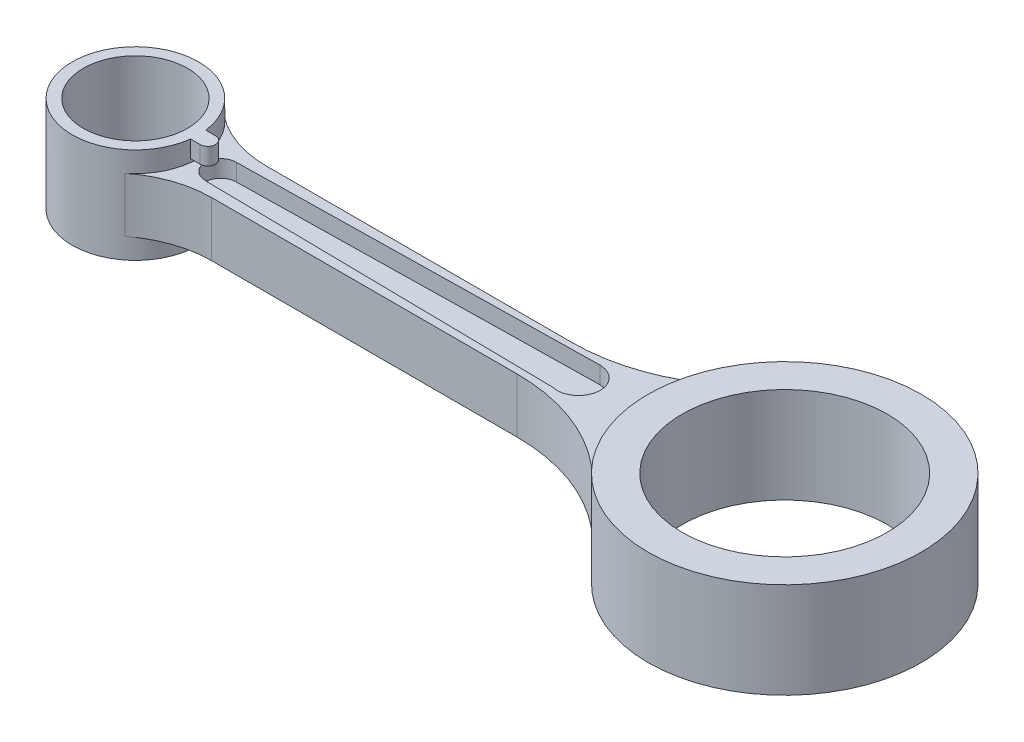
ISO-10303-21;
HEADER;
FILE_DESCRIPTION(('STEP AP214'),'2;1');
FILE_NAME('part.step','',(''),(''),'','','');
FILE_SCHEMA(('AUTOMOTIVE_DESIGN { 1 0 10303 214 1 1 1 1 }'));
ENDSEC;
DATA;
#1=APPLICATION_CONTEXT('core data for automotive mechanical design processes');
#2=APPLICATION_PROTOCOL_DEFINITION('international standard','automotive_design',2000,#1);
#3=PRODUCT_CONTEXT('',#1,'mechanical');
#4=PRODUCT('Part','Part','',(#3));
#5=PRODUCT_RELATED_PRODUCT_CATEGORY('part','',(#4));
#6=PRODUCT_DEFINITION_FORMATION('','',#4);
#7=PRODUCT_DEFINITION_CONTEXT('part definition',#1,'design');
#8=PRODUCT_DEFINITION('design','',#6,#7);
#9=PRODUCT_DEFINITION_SHAPE('','',#8);
#10=(LENGTH_UNIT() NAMED_UNIT(*) SI_UNIT(.MILLI.,.METRE.));
#11=(NAMED_UNIT(*) PLANE_ANGLE_UNIT() SI_UNIT($,.RADIAN.));
#12=(NAMED_UNIT(*) SI_UNIT($,.STERADIAN.) SOLID_ANGLE_UNIT());
#13=UNCERTAINTY_MEASURE_WITH_UNIT(LENGTH_MEASURE(1.E-05),#10,'distance_accuracy_value','');
#14=(GEOMETRIC_REPRESENTATION_CONTEXT(3) GLOBAL_UNCERTAINTY_ASSIGNED_CONTEXT((#13)) GLOBAL_UNIT_ASSIGNED_CONTEXT((#10,
#11,#12)) REPRESENTATION_CONTEXT('',''));
#15=CARTESIAN_POINT('',(0.,0.,0.));
#16=DIRECTION('',(0.,0.,1.));
#17=DIRECTION('',(1.,0.,0.));
#18=AXIS2_PLACEMENT_3D('',#15,#16,#17);
#19=CARTESIAN_POINT('',(12.3318325754668,7.,30.65));
#20=DIRECTION('',(0.,-1.,0.));
#21=DIRECTION('',(0.,0.,-1.));
#22=AXIS2_PLACEMENT_3D('',#19,#20,#21);
#23=CYLINDRICAL_SURFACE('',#22,26.65);
#24=DIRECTION('',(0.,1.,0.));
#25=VECTOR('',#24,1.);
#26=CARTESIAN_POINT('',(12.3318325754668,7.,4.));
#27=LINE('',#26,#25);
#28=CARTESIAN_POINT('',(12.3318325754668,-4.,4.));
#29=VERTEX_POINT('',#28);
#30=CARTESIAN_POINT('',(12.3318325754668,4.,4.));
#31=VERTEX_POINT('',#30);
#32=EDGE_CURVE('E337',#29,#31,#27,.T.);
#33=ORIENTED_EDGE('',*,*,#32,.F.);
#34=CARTESIAN_POINT('',(12.3318325754668,-4.,30.65));
#35=DIRECTION('',(0.,1.,0.));
#36=DIRECTION('',(0.,0.,1.));
#37=AXIS2_PLACEMENT_3D('',#34,#35,#36);
#38=CIRCLE('',#37,26.65);
#39=CARTESIAN_POINT('',(32.4225434407146,-4.,13.1404072883173));
#40=VERTEX_POINT('',#39);
#41=EDGE_CURVE('E341',#29,#40,#38,.F.);
#42=ORIENTED_EDGE('',*,*,#41,.T.);
#43=DIRECTION('',(0.,-1.,0.));
#44=VECTOR('',#43,1.);
#45=CARTESIAN_POINT('',(32.4225434407146,7.,13.1404072883173));
#46=LINE('',#45,#44);
#47=CARTESIAN_POINT('',(32.4225434407146,4.,13.1404072883173));
#48=VERTEX_POINT('',#47);
#49=EDGE_CURVE('E339',#48,#40,#46,.T.);
#50=ORIENTED_EDGE('',*,*,#49,.F.);
#51=CARTESIAN_POINT('',(12.3318325754668,4.,30.65));
#52=DIRECTION('',(0.,1.,0.));
#53=DIRECTION('',(0.,0.,1.));
#54=AXIS2_PLACEMENT_3D('',#51,#52,#53);
#55=CIRCLE('',#54,26.65);
#56=EDGE_CURVE('E48',#48,#31,#55,.T.);
#57=ORIENTED_EDGE('',*,*,#56,.T.);
#58=EDGE_LOOP('',(#33,#42,#50,#57));
#59=FACE_BOUND('',#58,.T.);
#60=ADVANCED_FACE('F41',(#59),#23,.F.);
#61=CARTESIAN_POINT('',(-32.3445554337723,7.,19.25));
#62=DIRECTION('',(0.,-1.,0.));
#63=DIRECTION('',(0.,0.,-1.));
#64=AXIS2_PLACEMENT_3D('',#61,#62,#63);
#65=CYLINDRICAL_SURFACE('',#64,15.25);
#66=DIRECTION('',(0.,-1.,0.));
#67=VECTOR('',#66,1.);
#68=CARTESIAN_POINT('',(-41.7780464392814,7.,7.26785714285715));
#69=LINE('',#68,#67);
#70=CARTESIAN_POINT('',(-41.7780464392814,-4.,7.26785714285715));
#71=VERTEX_POINT('',#70);
#72=CARTESIAN_POINT('',(-41.7780464392814,4.,7.26785714285715));
#73=VERTEX_POINT('',#72);
#74=EDGE_CURVE('E322',#71,#73,#69,.F.);
#75=ORIENTED_EDGE('',*,*,#74,.F.);
#76=CARTESIAN_POINT('',(-32.3445554337723,-4.,19.25));
#77=DIRECTION('',(0.,1.,0.));
#78=DIRECTION('',(0.,0.,1.));
#79=AXIS2_PLACEMENT_3D('',#76,#77,#78);
#80=CIRCLE('',#79,15.25);
#81=CARTESIAN_POINT('',(-32.3445554337723,-4.,4.));
#82=VERTEX_POINT('',#81);
#83=EDGE_CURVE('E334',#71,#82,#80,.F.);
#84=ORIENTED_EDGE('',*,*,#83,.T.);
#85=DIRECTION('',(0.,1.,0.));
#86=VECTOR('',#85,1.);
#87=CARTESIAN_POINT('',(-32.3445554337723,7.,4.));
#88=LINE('',#87,#86);
#89=CARTESIAN_POINT('',(-32.3445554337723,4.,4.));
#90=VERTEX_POINT('',#89);
#91=EDGE_CURVE('E330',#90,#82,#88,.F.);
#92=ORIENTED_EDGE('',*,*,#91,.F.);
#93=CARTESIAN_POINT('',(-32.3445554337723,4.,19.25));
#94=DIRECTION('',(0.,1.,0.));
#95=DIRECTION('',(0.,0.,1.));
#96=AXIS2_PLACEMENT_3D('',#93,#94,#95);
#97=CIRCLE('',#96,15.25);
#98=EDGE_CURVE('E335',#90,#73,#97,.T.);
#99=ORIENTED_EDGE('',*,*,#98,.T.);
#100=EDGE_LOOP('',(#75,#84,#92,#99));
#101=FACE_BOUND('',#100,.T.);
#102=ADVANCED_FACE('F356',(#101),#65,.F.);
#103=CARTESIAN_POINT('',(-32.3445554337723,7.,-19.25));
#104=DIRECTION('',(0.,-1.,0.));
#105=DIRECTION('',(0.,0.,-1.));
#106=AXIS2_PLACEMENT_3D('',#103,#104,#105);
#107=CYLINDRICAL_SURFACE('',#106,15.25);
#108=DIRECTION('',(0.,-1.,0.));
#109=VECTOR('',#108,1.);
#110=CARTESIAN_POINT('',(-41.7780464392814,7.,-7.26785714285714));
#111=LINE('',#110,#109);
#112=CARTESIAN_POINT('',(-41.7780464392814,4.,-7.26785714285714));
#113=VERTEX_POINT('',#112);
#114=CARTESIAN_POINT('',(-41.7780464392814,-4.,-7.26785714285714));
#115=VERTEX_POINT('',#114);
#116=EDGE_CURVE('E313',#113,#115,#111,.T.);
#117=ORIENTED_EDGE('',*,*,#116,.F.);
#118=CARTESIAN_POINT('',(-32.3445554337723,4.,-19.25));
#119=DIRECTION('',(0.,1.,0.));
#120=DIRECTION('',(0.,0.,1.));
#121=AXIS2_PLACEMENT_3D('',#118,#119,#120);
#122=CIRCLE('',#121,15.25);
#123=CARTESIAN_POINT('',(-32.3445554337723,4.,-4.));
#124=VERTEX_POINT('',#123);
#125=EDGE_CURVE('E318',#113,#124,#122,.T.);
#126=ORIENTED_EDGE('',*,*,#125,.T.);
#127=DIRECTION('',(0.,1.,0.));
#128=VECTOR('',#127,1.);
#129=CARTESIAN_POINT('',(-32.3445554337723,7.,-4.));
#130=LINE('',#129,#128);
#131=CARTESIAN_POINT('',(-32.3445554337723,-4.,-4.));
#132=VERTEX_POINT('',#131);
#133=EDGE_CURVE('E320',#132,#124,#130,.T.);
#134=ORIENTED_EDGE('',*,*,#133,.F.);
#135=CARTESIAN_POINT('',(-32.3445554337723,-4.,-19.25));
#136=DIRECTION('',(0.,1.,0.));
#137=DIRECTION('',(0.,0.,1.));
#138=AXIS2_PLACEMENT_3D('',#135,#136,#137);
#139=CIRCLE('',#138,15.25);
#140=EDGE_CURVE('E321',#132,#115,#139,.F.);
#141=ORIENTED_EDGE('',*,*,#140,.T.);
#142=EDGE_LOOP('',(#117,#126,#134,#141));
#143=FACE_BOUND('',#142,.T.);
#144=ADVANCED_FACE('F380',(#143),#107,.F.);
#145=CARTESIAN_POINT('',(12.3318325754668,7.,-30.65));
#146=DIRECTION('',(0.,-1.,0.));
#147=DIRECTION('',(0.,0.,-1.));
#148=AXIS2_PLACEMENT_3D('',#145,#146,#147);
#149=CYLINDRICAL_SURFACE('',#148,26.65);
#150=DIRECTION('',(0.,1.,0.));
#151=VECTOR('',#150,1.);
#152=CARTESIAN_POINT('',(12.3318325754668,7.,-4.));
#153=LINE('',#152,#151);
#154=CARTESIAN_POINT('',(12.3318325754668,4.,-4.));
#155=VERTEX_POINT('',#154);
#156=CARTESIAN_POINT('',(12.3318325754668,-4.,-4.));
#157=VERTEX_POINT('',#156);
#158=EDGE_CURVE('E303',#155,#157,#153,.F.);
#159=ORIENTED_EDGE('',*,*,#158,.F.);
#160=CARTESIAN_POINT('',(12.3318325754668,4.,-30.65));
#161=DIRECTION('',(0.,1.,0.));
#162=DIRECTION('',(0.,0.,1.));
#163=AXIS2_PLACEMENT_3D('',#160,#161,#162);
#164=CIRCLE('',#163,26.65);
#165=CARTESIAN_POINT('',(32.4225434407146,4.,-13.1404072883173));
#166=VERTEX_POINT('',#165);
#167=EDGE_CURVE('E307',#155,#166,#164,.T.);
#168=ORIENTED_EDGE('',*,*,#167,.T.);
#169=DIRECTION('',(0.,-1.,0.));
#170=VECTOR('',#169,1.);
#171=CARTESIAN_POINT('',(32.4225434407146,7.,-13.1404072883173));
#172=LINE('',#171,#170);
#173=CARTESIAN_POINT('',(32.4225434407146,-4.,-13.1404072883173));
#174=VERTEX_POINT('',#173);
#175=EDGE_CURVE('E306',#174,#166,#172,.F.);
#176=ORIENTED_EDGE('',*,*,#175,.F.);
#177=CARTESIAN_POINT('',(12.3318325754668,-4.,-30.65));
#178=DIRECTION('',(0.,1.,0.));
#179=DIRECTION('',(0.,0.,1.));
#180=AXIS2_PLACEMENT_3D('',#177,#178,#179);
#181=CIRCLE('',#180,26.65);
#182=EDGE_CURVE('E315',#174,#157,#181,.F.);
#183=ORIENTED_EDGE('',*,*,#182,.T.);
#184=EDGE_LOOP('',(#159,#168,#176,#183));
#185=FACE_BOUND('',#184,.T.);
#186=ADVANCED_FACE('F367',(#185),#149,.F.);
#187=CARTESIAN_POINT('',(-38.3065183264543,4.,4.));
#188=DIRECTION('',(0.,0.,-1.));
#189=DIRECTION('',(-1.,0.,0.));
#190=AXIS2_PLACEMENT_3D('',#187,#188,#189);
#191=PLANE('',#190);
#192=DIRECTION('',(1.,0.,0.));
#193=VECTOR('',#192,1.);
#194=CARTESIAN_POINT('',(-38.3065183264543,-4.,4.));
#195=LINE('',#194,#193);
#196=EDGE_CURVE('E271',#82,#29,#195,.T.);
#197=ORIENTED_EDGE('',*,*,#196,.T.);
#198=ORIENTED_EDGE('',*,*,#32,.T.);
#199=DIRECTION('',(1.,0.,0.));
#200=VECTOR('',#199,1.);
#201=CARTESIAN_POINT('',(-39.3751793252666,4.,4.));
#202=LINE('',#201,#200);
#203=EDGE_CURVE('E274',#90,#31,#202,.T.);
#204=ORIENTED_EDGE('',*,*,#203,.F.);
#205=ORIENTED_EDGE('',*,*,#91,.T.);
#206=EDGE_LOOP('',(#197,#198,#204,#205));
#207=FACE_BOUND('',#206,.T.);
#208=ADVANCED_FACE('F354',(#207),#191,.F.);
#209=CARTESIAN_POINT('',(27.2825504756529,4.,-4.));
#210=DIRECTION('',(0.,0.,1.));
#211=DIRECTION('',(1.,0.,0.));
#212=AXIS2_PLACEMENT_3D('',#209,#210,#211);
#213=PLANE('',#212);
#214=DIRECTION('',(-1.,0.,0.));
#215=VECTOR('',#214,1.);
#216=CARTESIAN_POINT('',(27.2825504756529,-4.,-4.));
#217=LINE('',#216,#215);
#218=EDGE_CURVE('E280',#157,#132,#217,.T.);
#219=ORIENTED_EDGE('',*,*,#218,.T.);
#220=ORIENTED_EDGE('',*,*,#133,.T.);
#221=DIRECTION('',(-1.,0.,0.));
#222=VECTOR('',#221,1.);
#223=CARTESIAN_POINT('',(27.2825504756529,4.,-4.));
#224=LINE('',#223,#222);
#225=EDGE_CURVE('E276',#155,#124,#224,.T.);
#226=ORIENTED_EDGE('',*,*,#225,.F.);
#227=ORIENTED_EDGE('',*,*,#158,.T.);
#228=EDGE_LOOP('',(#219,#220,#226,#227));
#229=FACE_BOUND('',#228,.T.);
#230=ADVANCED_FACE('F373',(#229),#213,.F.);
#231=CARTESIAN_POINT('',(47.5,7.,0.));
#232=DIRECTION('',(0.,-1.,0.));
#233=DIRECTION('',(0.,0.,-1.));
#234=AXIS2_PLACEMENT_3D('',#231,#232,#233);
#235=CYLINDRICAL_SURFACE('',#234,15.);
#236=CARTESIAN_POINT('',(47.5,7.,0.));
#237=DIRECTION('',(0.,1.,0.));
#238=DIRECTION('',(0.,0.,1.));
#239=AXIS2_PLACEMENT_3D('',#236,#237,#238);
#240=CIRCLE('',#239,15.);
#241=CARTESIAN_POINT('',(47.5,7.,15.));
#242=VERTEX_POINT('',#241);
#243=EDGE_CURVE('E289',#242,#242,#240,.T.);
#244=ORIENTED_EDGE('',*,*,#243,.T.);
#245=EDGE_LOOP('',(#244));
#246=FACE_BOUND('',#245,.T.);
#247=CARTESIAN_POINT('',(47.5,-7.,0.));
#248=DIRECTION('',(0.,1.,0.));
#249=DIRECTION('',(0.,0.,1.));
#250=AXIS2_PLACEMENT_3D('',#247,#248,#249);
#251=CIRCLE('',#250,15.);
#252=CARTESIAN_POINT('',(47.5,-7.,15.));
#253=VERTEX_POINT('',#252);
#254=EDGE_CURVE('E282',#253,#253,#251,.T.);
#255=ORIENTED_EDGE('',*,*,#254,.F.);
#256=EDGE_LOOP('',(#255));
#257=FACE_BOUND('',#256,.T.);
#258=ADVANCED_FACE('F411',(#246,#257),#235,.F.);
#259=CARTESIAN_POINT('',(47.5,7.,0.));
#260=DIRECTION('',(0.,-1.,0.));
#261=DIRECTION('',(0.,0.,-1.));
#262=AXIS2_PLACEMENT_3D('',#259,#260,#261);
#263=CYLINDRICAL_SURFACE('',#262,20.);
#264=ORIENTED_EDGE('',*,*,#49,.T.);
#265=CARTESIAN_POINT('',(47.5,-4.,0.));
#266=DIRECTION('',(0.,1.,0.));
#267=DIRECTION('',(0.,0.,1.));
#268=AXIS2_PLACEMENT_3D('',#265,#266,#267);
#269=CIRCLE('',#268,20.);
#270=EDGE_CURVE('E291',#174,#40,#269,.T.);
#271=ORIENTED_EDGE('',*,*,#270,.F.);
#272=ORIENTED_EDGE('',*,*,#175,.T.);
#273=CARTESIAN_POINT('',(47.5,4.,0.));
#274=DIRECTION('',(0.,1.,0.));
#275=DIRECTION('',(0.,0.,1.));
#276=AXIS2_PLACEMENT_3D('',#273,#274,#275);
#277=CIRCLE('',#276,20.);
#278=EDGE_CURVE('E299',#166,#48,#277,.T.);
#279=ORIENTED_EDGE('',*,*,#278,.T.);
#280=EDGE_LOOP('',(#264,#271,#272,#279));
#281=FACE_BOUND('',#280,.T.);
#282=CARTESIAN_POINT('',(47.5,7.,0.));
#283=DIRECTION('',(0.,1.,0.));
#284=DIRECTION('',(0.,0.,1.));
#285=AXIS2_PLACEMENT_3D('',#282,#283,#284);
#286=CIRCLE('',#285,20.);
#287=CARTESIAN_POINT('',(47.5,7.,20.));
#288=VERTEX_POINT('',#287);
#289=EDGE_CURVE('E288',#288,#288,#286,.T.);
#290=ORIENTED_EDGE('',*,*,#289,.F.);
#291=EDGE_LOOP('',(#290));
#292=FACE_BOUND('',#291,.T.);
#293=CARTESIAN_POINT('',(47.5,-7.,0.));
#294=DIRECTION('',(0.,1.,0.));
#295=DIRECTION('',(0.,0.,1.));
#296=AXIS2_PLACEMENT_3D('',#293,#294,#295);
#297=CIRCLE('',#296,20.);
#298=CARTESIAN_POINT('',(47.5,-7.,20.));
#299=VERTEX_POINT('',#298);
#300=EDGE_CURVE('E287',#299,#299,#297,.T.);
#301=ORIENTED_EDGE('',*,*,#300,.T.);
#302=EDGE_LOOP('',(#301));
#303=FACE_BOUND('',#302,.T.);
#304=ADVANCED_FACE('F364',(#281,#292,#303),#263,.T.);
#305=CARTESIAN_POINT('',(0.,7.,0.));
#306=DIRECTION('',(0.,1.,0.));
#307=DIRECTION('',(0.,0.,1.));
#308=AXIS2_PLACEMENT_3D('',#305,#306,#307);
#309=PLANE('',#308);
#310=ORIENTED_EDGE('',*,*,#243,.F.);
#311=EDGE_LOOP('',(#310));
#312=FACE_BOUND('',#311,.T.);
#313=ORIENTED_EDGE('',*,*,#289,.T.);
#314=EDGE_LOOP('',(#313));
#315=FACE_BOUND('',#314,.T.);
#316=ADVANCED_FACE('F417',(#312,#315),#309,.T.);
#317=CARTESIAN_POINT('',(0.,-7.,0.));
#318=DIRECTION('',(0.,1.,0.));
#319=DIRECTION('',(0.,0.,1.));
#320=AXIS2_PLACEMENT_3D('',#317,#318,#319);
#321=PLANE('',#320);
#322=ORIENTED_EDGE('',*,*,#254,.T.);
#323=EDGE_LOOP('',(#322));
#324=FACE_BOUND('',#323,.T.);
#325=ORIENTED_EDGE('',*,*,#300,.F.);
#326=EDGE_LOOP('',(#325));
#327=FACE_BOUND('',#326,.T.);
#328=ADVANCED_FACE('F423',(#324,#327),#321,.F.);
#329=CARTESIAN_POINT('',(0.,4.,0.));
#330=DIRECTION('',(0.,1.,0.));
#331=DIRECTION('',(0.,0.,1.));
#332=AXIS2_PLACEMENT_3D('',#329,#330,#331);
#333=PLANE('',#332);
#334=DIRECTION('',(0.999892618853564,0.,0.0146543768943431));
#335=VECTOR('',#334,1.);
#336=CARTESIAN_POINT('',(-0.0414886671393151,4.,2.8308410748387));
#337=LINE('',#336,#335);
#338=CARTESIAN_POINT('',(-35.01,4.,2.31834429784139));
#339=VERTEX_POINT('',#338);
#340=CARTESIAN_POINT('',(16.5719942554758,4.,3.07432746096172));
#341=VERTEX_POINT('',#340);
#342=EDGE_CURVE('E65',#339,#341,#337,.T.);
#343=ORIENTED_EDGE('',*,*,#342,.F.);
#344=DIRECTION('',(0.,0.,1.));
#345=VECTOR('',#344,1.);
#346=CARTESIAN_POINT('',(-35.01,4.,0.));
#347=LINE('',#346,#345);
#348=CARTESIAN_POINT('',(-35.01,4.,2.27758375371882));
#349=VERTEX_POINT('',#348);
#350=EDGE_CURVE('E208',#349,#339,#347,.T.);
#351=ORIENTED_EDGE('',*,*,#350,.F.);
#352=CARTESIAN_POINT('',(-35.01,4.,0.));
#353=DIRECTION('',(0.,1.,0.));
#354=DIRECTION('',(0.,0.,1.));
#355=AXIS2_PLACEMENT_3D('',#352,#353,#354);
#356=CIRCLE('',#355,2.27758375371882);
#357=CARTESIAN_POINT('',(-35.01,4.,-2.27758375371881));
#358=VERTEX_POINT('',#357);
#359=EDGE_CURVE('E245',#358,#349,#356,.T.);
#360=ORIENTED_EDGE('',*,*,#359,.F.);
#361=DIRECTION('',(0.,0.,1.));
#362=VECTOR('',#361,1.);
#363=CARTESIAN_POINT('',(-35.01,4.,0.));
#364=LINE('',#363,#362);
#365=CARTESIAN_POINT('',(-35.01,4.,-2.28421044966346));
#366=VERTEX_POINT('',#365);
#367=EDGE_CURVE('E237',#366,#358,#364,.T.);
#368=ORIENTED_EDGE('',*,*,#367,.F.);
#369=DIRECTION('',(-0.99985003095603,0.,0.0173180714060757));
#370=VECTOR('',#369,1.);
#371=CARTESIAN_POINT('',(-0.0500522322392675,4.,-2.8897401321658));
#372=LINE('',#371,#370);
#373=CARTESIAN_POINT('',(17.33,4.,-3.19077426356593));
#374=VERTEX_POINT('',#373);
#375=EDGE_CURVE('E236',#374,#366,#372,.T.);
#376=ORIENTED_EDGE('',*,*,#375,.F.);
#377=DIRECTION('',(0.,0.,-1.));
#378=VECTOR('',#377,1.);
#379=CARTESIAN_POINT('',(17.33,4.,0.));
#380=LINE('',#379,#378);
#381=CARTESIAN_POINT('',(17.33,4.,-3.1663957500532));
#382=VERTEX_POINT('',#381);
#383=EDGE_CURVE('E231',#382,#374,#380,.T.);
#384=ORIENTED_EDGE('',*,*,#383,.F.);
#385=CARTESIAN_POINT('',(17.33,4.,0.));
#386=DIRECTION('',(0.,1.,0.));
#387=DIRECTION('',(0.,0.,1.));
#388=AXIS2_PLACEMENT_3D('',#385,#386,#387);
#389=CIRCLE('',#388,3.1663957500532);
#390=EDGE_CURVE('E229',#341,#382,#389,.T.);
#391=ORIENTED_EDGE('',*,*,#390,.F.);
#392=EDGE_LOOP('',(#343,#351,#360,#368,#376,#384,#391));
#393=FACE_BOUND('',#392,.T.);
#394=ORIENTED_EDGE('',*,*,#278,.F.);
#395=ORIENTED_EDGE('',*,*,#167,.F.);
#396=ORIENTED_EDGE('',*,*,#225,.T.);
#397=ORIENTED_EDGE('',*,*,#125,.F.);
#398=CARTESIAN_POINT('',(-47.5,4.,0.));
#399=DIRECTION('',(0.,1.,0.));
#400=DIRECTION('',(0.,0.,1.));
#401=AXIS2_PLACEMENT_3D('',#398,#399,#400);
#402=CIRCLE('',#401,9.25);
#403=EDGE_CURVE('E266',#113,#73,#402,.F.);
#404=ORIENTED_EDGE('',*,*,#403,.T.);
#405=ORIENTED_EDGE('',*,*,#98,.F.);
#406=ORIENTED_EDGE('',*,*,#203,.T.);
#407=ORIENTED_EDGE('',*,*,#56,.F.);
#408=EDGE_LOOP('',(#394,#395,#396,#397,#404,#405,#406,#407));
#409=FACE_BOUND('',#408,.T.);
#410=ADVANCED_FACE('F355',(#393,#409),#333,.T.);
#411=CARTESIAN_POINT('',(0.,-4.,0.));
#412=DIRECTION('',(0.,1.,0.));
#413=DIRECTION('',(0.,0.,1.));
#414=AXIS2_PLACEMENT_3D('',#411,#412,#413);
#415=PLANE('',#414);
#416=CARTESIAN_POINT('',(-47.5,-4.,0.));
#417=DIRECTION('',(0.,1.,0.));
#418=DIRECTION('',(0.,0.,1.));
#419=AXIS2_PLACEMENT_3D('',#416,#417,#418);
#420=CIRCLE('',#419,9.25);
#421=EDGE_CURVE('E301',#115,#71,#420,.F.);
#422=ORIENTED_EDGE('',*,*,#421,.F.);
#423=ORIENTED_EDGE('',*,*,#140,.F.);
#424=ORIENTED_EDGE('',*,*,#218,.F.);
#425=ORIENTED_EDGE('',*,*,#182,.F.);
#426=ORIENTED_EDGE('',*,*,#270,.T.);
#427=ORIENTED_EDGE('',*,*,#41,.F.);
#428=ORIENTED_EDGE('',*,*,#196,.F.);
#429=ORIENTED_EDGE('',*,*,#83,.F.);
#430=EDGE_LOOP('',(#422,#423,#424,#425,#426,#427,#428,#429));
#431=FACE_BOUND('',#430,.T.);
#432=ADVANCED_FACE('F363',(#431),#415,.F.);
#433=CARTESIAN_POINT('',(-47.5,7.,0.));
#434=DIRECTION('',(0.,-1.,0.));
#435=DIRECTION('',(0.,0.,-1.));
#436=AXIS2_PLACEMENT_3D('',#433,#434,#435);
#437=CYLINDRICAL_SURFACE('',#436,7.625);
#438=CARTESIAN_POINT('',(-47.5,7.,0.));
#439=DIRECTION('',(0.,1.,0.));
#440=DIRECTION('',(0.,0.,1.));
#441=AXIS2_PLACEMENT_3D('',#438,#439,#440);
#442=CIRCLE('',#441,7.625);
#443=CARTESIAN_POINT('',(-47.5,7.,7.62500000000001));
#444=VERTEX_POINT('',#443);
#445=EDGE_CURVE('E262',#444,#444,#442,.T.);
#446=ORIENTED_EDGE('',*,*,#445,.T.);
#447=EDGE_LOOP('',(#446));
#448=FACE_BOUND('',#447,.T.);
#449=CARTESIAN_POINT('',(-47.5,-7.,0.));
#450=DIRECTION('',(0.,1.,0.));
#451=DIRECTION('',(0.,0.,1.));
#452=AXIS2_PLACEMENT_3D('',#449,#450,#451);
#453=CIRCLE('',#452,7.625);
#454=CARTESIAN_POINT('',(-47.5,-7.,7.62500000000001));
#455=VERTEX_POINT('',#454);
#456=EDGE_CURVE('E248',#455,#455,#453,.T.);
#457=ORIENTED_EDGE('',*,*,#456,.F.);
#458=EDGE_LOOP('',(#457));
#459=FACE_BOUND('',#458,.T.);
#460=ADVANCED_FACE('F384',(#448,#459),#437,.F.);
#461=CARTESIAN_POINT('',(-47.5,7.,0.));
#462=DIRECTION('',(0.,-1.,0.));
#463=DIRECTION('',(0.,0.,-1.));
#464=AXIS2_PLACEMENT_3D('',#461,#462,#463);
#465=CYLINDRICAL_SURFACE('',#464,9.25);
#466=CARTESIAN_POINT('',(-47.5,7.,0.));
#467=DIRECTION('',(0.,1.,0.));
#468=DIRECTION('',(0.,0.,1.));
#469=AXIS2_PLACEMENT_3D('',#466,#467,#468);
#470=CIRCLE('',#469,9.25);
#471=CARTESIAN_POINT('',(-38.3174472503557,7.,-1.115));
#472=VERTEX_POINT('',#471);
#473=CARTESIAN_POINT('',(-38.3174472503557,7.,1.115));
#474=VERTEX_POINT('',#473);
#475=EDGE_CURVE('E261',#472,#474,#470,.T.);
#476=ORIENTED_EDGE('',*,*,#475,.F.);
#477=DIRECTION('',(0.,-1.,0.));
#478=VECTOR('',#477,1.);
#479=CARTESIAN_POINT('',(-38.3174472503557,7.,-1.115));
#480=LINE('',#479,#478);
#481=CARTESIAN_POINT('',(-38.3174472503557,4.5,-1.115));
#482=VERTEX_POINT('',#481);
#483=EDGE_CURVE('E205',#472,#482,#480,.T.);
#484=ORIENTED_EDGE('',*,*,#483,.T.);
#485=CARTESIAN_POINT('',(-47.5,4.5,0.));
#486=DIRECTION('',(0.,1.,0.));
#487=DIRECTION('',(0.,0.,1.));
#488=AXIS2_PLACEMENT_3D('',#485,#486,#487);
#489=CIRCLE('',#488,9.25);
#490=CARTESIAN_POINT('',(-38.3174472503557,4.5,1.115));
#491=VERTEX_POINT('',#490);
#492=EDGE_CURVE('E11',#491,#482,#489,.T.);
#493=ORIENTED_EDGE('',*,*,#492,.F.);
#494=DIRECTION('',(0.,-1.,0.));
#495=VECTOR('',#494,1.);
#496=CARTESIAN_POINT('',(-38.3174472503557,7.,1.115));
#497=LINE('',#496,#495);
#498=EDGE_CURVE('E178',#491,#474,#497,.F.);
#499=ORIENTED_EDGE('',*,*,#498,.T.);
#500=EDGE_LOOP('',(#476,#484,#493,#499));
#501=FACE_BOUND('',#500,.T.);
#502=ORIENTED_EDGE('',*,*,#421,.T.);
#503=ORIENTED_EDGE('',*,*,#74,.T.);
#504=ORIENTED_EDGE('',*,*,#403,.F.);
#505=ORIENTED_EDGE('',*,*,#116,.T.);
#506=EDGE_LOOP('',(#502,#503,#504,#505));
#507=FACE_BOUND('',#506,.T.);
#508=CARTESIAN_POINT('',(-47.5,-7.,0.));
#509=DIRECTION('',(0.,1.,0.));
#510=DIRECTION('',(0.,0.,1.));
#511=AXIS2_PLACEMENT_3D('',#508,#509,#510);
#512=CIRCLE('',#511,9.25);
#513=CARTESIAN_POINT('',(-47.5,-7.,9.25000000000001));
#514=VERTEX_POINT('',#513);
#515=EDGE_CURVE('E263',#514,#514,#512,.T.);
#516=ORIENTED_EDGE('',*,*,#515,.T.);
#517=EDGE_LOOP('',(#516));
#518=FACE_BOUND('',#517,.T.);
#519=ADVANCED_FACE('F378',(#501,#507,#518),#465,.T.);
#520=CARTESIAN_POINT('',(0.,7.,0.));
#521=DIRECTION('',(0.,1.,0.));
#522=DIRECTION('',(0.,0.,1.));
#523=AXIS2_PLACEMENT_3D('',#520,#521,#522);
#524=PLANE('',#523);
#525=ORIENTED_EDGE('',*,*,#475,.T.);
#526=DIRECTION('',(1.,0.,0.));
#527=VECTOR('',#526,1.);
#528=CARTESIAN_POINT('',(0.,7.,1.115));
#529=LINE('',#528,#527);
#530=CARTESIAN_POINT('',(-36.9060551700783,7.,1.115));
#531=VERTEX_POINT('',#530);
#532=EDGE_CURVE('E199',#474,#531,#529,.T.);
#533=ORIENTED_EDGE('',*,*,#532,.T.);
#534=CARTESIAN_POINT('',(-36.9060551700783,7.,0.));
#535=DIRECTION('',(0.,1.,0.));
#536=DIRECTION('',(0.,0.,1.));
#537=AXIS2_PLACEMENT_3D('',#534,#535,#536);
#538=CIRCLE('',#537,1.115);
#539=CARTESIAN_POINT('',(-36.9060551700783,7.,-1.115));
#540=VERTEX_POINT('',#539);
#541=EDGE_CURVE('E189',#531,#540,#538,.T.);
#542=ORIENTED_EDGE('',*,*,#541,.T.);
#543=DIRECTION('',(-1.,0.,0.));
#544=VECTOR('',#543,1.);
#545=CARTESIAN_POINT('',(0.,7.,-1.115));
#546=LINE('',#545,#544);
#547=EDGE_CURVE('E54',#540,#472,#546,.T.);
#548=ORIENTED_EDGE('',*,*,#547,.T.);
#549=EDGE_LOOP('',(#525,#533,#542,#548));
#550=FACE_BOUND('',#549,.T.);
#551=ORIENTED_EDGE('',*,*,#445,.F.);
#552=EDGE_LOOP('',(#551));
#553=FACE_BOUND('',#552,.T.);
#554=ADVANCED_FACE('F385',(#550,#553),#524,.T.);
#555=CARTESIAN_POINT('',(0.,-7.,0.));
#556=DIRECTION('',(0.,1.,0.));
#557=DIRECTION('',(0.,0.,1.));
#558=AXIS2_PLACEMENT_3D('',#555,#556,#557);
#559=PLANE('',#558);
#560=ORIENTED_EDGE('',*,*,#456,.T.);
#561=EDGE_LOOP('',(#560));
#562=FACE_BOUND('',#561,.T.);
#563=ORIENTED_EDGE('',*,*,#515,.F.);
#564=EDGE_LOOP('',(#563));
#565=FACE_BOUND('',#564,.T.);
#566=ADVANCED_FACE('F390',(#562,#565),#559,.F.);
#567=CARTESIAN_POINT('',(-0.0414886671393151,1.5,2.8308410748387));
#568=DIRECTION('',(-0.0146543768943431,0.,0.999892618853564));
#569=DIRECTION('',(0.999892618853564,0.,0.0146543768943431));
#570=AXIS2_PLACEMENT_3D('',#567,#568,#569);
#571=PLANE('',#570);
#572=ORIENTED_EDGE('',*,*,#342,.T.);
#573=DIRECTION('',(0.,1.,0.));
#574=VECTOR('',#573,1.);
#575=CARTESIAN_POINT('',(16.5719942554758,1.5,3.07432746096172));
#576=LINE('',#575,#574);
#577=CARTESIAN_POINT('',(16.5719942554758,1.5,3.07432746096172));
#578=VERTEX_POINT('',#577);
#579=EDGE_CURVE('E226',#578,#341,#576,.T.);
#580=ORIENTED_EDGE('',*,*,#579,.F.);
#581=DIRECTION('',(0.999892618853564,0.,0.0146543768943431));
#582=VECTOR('',#581,1.);
#583=CARTESIAN_POINT('',(-0.0414886671393151,1.5,2.8308410748387));
#584=LINE('',#583,#582);
#585=CARTESIAN_POINT('',(-35.01,1.5,2.31834429784139));
#586=VERTEX_POINT('',#585);
#587=EDGE_CURVE('E207',#586,#578,#584,.T.);
#588=ORIENTED_EDGE('',*,*,#587,.F.);
#589=DIRECTION('',(0.,1.,0.));
#590=VECTOR('',#589,1.);
#591=CARTESIAN_POINT('',(-35.01,1.5,2.31834429784139));
#592=LINE('',#591,#590);
#593=EDGE_CURVE('E250',#586,#339,#592,.T.);
#594=ORIENTED_EDGE('',*,*,#593,.T.);
#595=EDGE_LOOP('',(#572,#580,#588,#594));
#596=FACE_BOUND('',#595,.T.);
#597=ADVANCED_FACE('F387',(#596),#571,.F.);
#598=CARTESIAN_POINT('',(-35.01,1.5,0.));
#599=DIRECTION('',(-1.,0.,0.));
#600=DIRECTION('',(0.,0.,1.));
#601=AXIS2_PLACEMENT_3D('',#598,#599,#600);
#602=PLANE('',#601);
#603=ORIENTED_EDGE('',*,*,#350,.T.);
#604=ORIENTED_EDGE('',*,*,#593,.F.);
#605=DIRECTION('',(0.,0.,1.));
#606=VECTOR('',#605,1.);
#607=CARTESIAN_POINT('',(-35.01,1.5,0.));
#608=LINE('',#607,#606);
#609=CARTESIAN_POINT('',(-35.01,1.5,2.27758375371882));
#610=VERTEX_POINT('',#609);
#611=EDGE_CURVE('E222',#610,#586,#608,.T.);
#612=ORIENTED_EDGE('',*,*,#611,.F.);
#613=DIRECTION('',(0.,1.,0.));
#614=VECTOR('',#613,1.);
#615=CARTESIAN_POINT('',(-35.01,1.5,2.27758375371882));
#616=LINE('',#615,#614);
#617=EDGE_CURVE('E249',#610,#349,#616,.T.);
#618=ORIENTED_EDGE('',*,*,#617,.T.);
#619=EDGE_LOOP('',(#603,#604,#612,#618));
#620=FACE_BOUND('',#619,.T.);
#621=ADVANCED_FACE('F400',(#620),#602,.F.);
#622=CARTESIAN_POINT('',(-35.01,1.5,0.));
#623=DIRECTION('',(0.,1.,0.));
#624=DIRECTION('',(0.,0.,1.));
#625=AXIS2_PLACEMENT_3D('',#622,#623,#624);
#626=CYLINDRICAL_SURFACE('',#625,2.27758375371882);
#627=ORIENTED_EDGE('',*,*,#359,.T.);
#628=ORIENTED_EDGE('',*,*,#617,.F.);
#629=CARTESIAN_POINT('',(-35.01,1.5,0.));
#630=DIRECTION('',(0.,1.,0.));
#631=DIRECTION('',(0.,0.,1.));
#632=AXIS2_PLACEMENT_3D('',#629,#630,#631);
#633=CIRCLE('',#632,2.27758375371882);
#634=CARTESIAN_POINT('',(-35.01,1.5,-2.27758375371881));
#635=VERTEX_POINT('',#634);
#636=EDGE_CURVE('E221',#635,#610,#633,.T.);
#637=ORIENTED_EDGE('',*,*,#636,.F.);
#638=DIRECTION('',(0.,1.,0.));
#639=VECTOR('',#638,1.);
#640=CARTESIAN_POINT('',(-35.01,1.5,-2.27758375371881));
#641=LINE('',#640,#639);
#642=EDGE_CURVE('E255',#635,#358,#641,.T.);
#643=ORIENTED_EDGE('',*,*,#642,.T.);
#644=EDGE_LOOP('',(#627,#628,#637,#643));
#645=FACE_BOUND('',#644,.T.);
#646=ADVANCED_FACE('F489',(#645),#626,.F.);
#647=CARTESIAN_POINT('',(-35.01,1.5,0.));
#648=DIRECTION('',(-1.,0.,0.));
#649=DIRECTION('',(0.,0.,1.));
#650=AXIS2_PLACEMENT_3D('',#647,#648,#649);
#651=PLANE('',#650);
#652=ORIENTED_EDGE('',*,*,#367,.T.);
#653=ORIENTED_EDGE('',*,*,#642,.F.);
#654=DIRECTION('',(0.,0.,1.));
#655=VECTOR('',#654,1.);
#656=CARTESIAN_POINT('',(-35.01,1.5,0.));
#657=LINE('',#656,#655);
#658=CARTESIAN_POINT('',(-35.01,1.5,-2.28421044966346));
#659=VERTEX_POINT('',#658);
#660=EDGE_CURVE('E216',#659,#635,#657,.T.);
#661=ORIENTED_EDGE('',*,*,#660,.F.);
#662=DIRECTION('',(0.,1.,0.));
#663=VECTOR('',#662,1.);
#664=CARTESIAN_POINT('',(-35.01,1.5,-2.28421044966346));
#665=LINE('',#664,#663);
#666=EDGE_CURVE('E251',#659,#366,#665,.T.);
#667=ORIENTED_EDGE('',*,*,#666,.T.);
#668=EDGE_LOOP('',(#652,#653,#661,#667));
#669=FACE_BOUND('',#668,.T.);
#670=ADVANCED_FACE('F497',(#669),#651,.F.);
#671=CARTESIAN_POINT('',(-0.0500522322392675,1.5,-2.8897401321658));
#672=DIRECTION('',(-0.0173180714060757,0.,-0.99985003095603));
#673=DIRECTION('',(-0.99985003095603,0.,0.0173180714060757));
#674=AXIS2_PLACEMENT_3D('',#671,#672,#673);
#675=PLANE('',#674);
#676=ORIENTED_EDGE('',*,*,#375,.T.);
#677=ORIENTED_EDGE('',*,*,#666,.F.);
#678=DIRECTION('',(-0.99985003095603,0.,0.0173180714060757));
#679=VECTOR('',#678,1.);
#680=CARTESIAN_POINT('',(-0.0500522322392675,1.5,-2.8897401321658));
#681=LINE('',#680,#679);
#682=CARTESIAN_POINT('',(17.33,1.5,-3.19077426356593));
#683=VERTEX_POINT('',#682);
#684=EDGE_CURVE('E217',#683,#659,#681,.T.);
#685=ORIENTED_EDGE('',*,*,#684,.F.);
#686=DIRECTION('',(0.,1.,0.));
#687=VECTOR('',#686,1.);
#688=CARTESIAN_POINT('',(17.33,1.5,-3.19077426356593));
#689=LINE('',#688,#687);
#690=EDGE_CURVE('E259',#683,#374,#689,.T.);
#691=ORIENTED_EDGE('',*,*,#690,.T.);
#692=EDGE_LOOP('',(#676,#677,#685,#691));
#693=FACE_BOUND('',#692,.T.);
#694=ADVANCED_FACE('F507',(#693),#675,.F.);
#695=CARTESIAN_POINT('',(17.33,1.5,0.));
#696=DIRECTION('',(1.,0.,0.));
#697=DIRECTION('',(0.,0.,-1.));
#698=AXIS2_PLACEMENT_3D('',#695,#696,#697);
#699=PLANE('',#698);
#700=ORIENTED_EDGE('',*,*,#383,.T.);
#701=ORIENTED_EDGE('',*,*,#690,.F.);
#702=DIRECTION('',(0.,0.,-1.));
#703=VECTOR('',#702,1.);
#704=CARTESIAN_POINT('',(17.33,1.5,0.));
#705=LINE('',#704,#703);
#706=CARTESIAN_POINT('',(17.33,1.5,-3.1663957500532));
#707=VERTEX_POINT('',#706);
#708=EDGE_CURVE('E215',#707,#683,#705,.T.);
#709=ORIENTED_EDGE('',*,*,#708,.F.);
#710=DIRECTION('',(0.,1.,0.));
#711=VECTOR('',#710,1.);
#712=CARTESIAN_POINT('',(17.33,1.5,-3.1663957500532));
#713=LINE('',#712,#711);
#714=EDGE_CURVE('E260',#707,#382,#713,.T.);
#715=ORIENTED_EDGE('',*,*,#714,.T.);
#716=EDGE_LOOP('',(#700,#701,#709,#715));
#717=FACE_BOUND('',#716,.T.);
#718=ADVANCED_FACE('F516',(#717),#699,.F.);
#719=CARTESIAN_POINT('',(17.33,1.5,0.));
#720=DIRECTION('',(0.,1.,0.));
#721=DIRECTION('',(0.,0.,1.));
#722=AXIS2_PLACEMENT_3D('',#719,#720,#721);
#723=CYLINDRICAL_SURFACE('',#722,3.1663957500532);
#724=ORIENTED_EDGE('',*,*,#390,.T.);
#725=ORIENTED_EDGE('',*,*,#714,.F.);
#726=CARTESIAN_POINT('',(17.33,1.5,0.));
#727=DIRECTION('',(0.,1.,0.));
#728=DIRECTION('',(0.,0.,1.));
#729=AXIS2_PLACEMENT_3D('',#726,#727,#728);
#730=CIRCLE('',#729,3.1663957500532);
#731=EDGE_CURVE('E209',#578,#707,#730,.T.);
#732=ORIENTED_EDGE('',*,*,#731,.F.);
#733=ORIENTED_EDGE('',*,*,#579,.T.);
#734=EDGE_LOOP('',(#724,#725,#732,#733));
#735=FACE_BOUND('',#734,.T.);
#736=ADVANCED_FACE('F529',(#735),#723,.F.);
#737=CARTESIAN_POINT('',(0.,1.5,0.));
#738=DIRECTION('',(0.,1.,0.));
#739=DIRECTION('',(0.,0.,1.));
#740=AXIS2_PLACEMENT_3D('',#737,#738,#739);
#741=PLANE('',#740);
#742=ORIENTED_EDGE('',*,*,#587,.T.);
#743=ORIENTED_EDGE('',*,*,#731,.T.);
#744=ORIENTED_EDGE('',*,*,#708,.T.);
#745=ORIENTED_EDGE('',*,*,#684,.T.);
#746=ORIENTED_EDGE('',*,*,#660,.T.);
#747=ORIENTED_EDGE('',*,*,#636,.T.);
#748=ORIENTED_EDGE('',*,*,#611,.T.);
#749=EDGE_LOOP('',(#742,#743,#744,#745,#746,#747,#748));
#750=FACE_BOUND('',#749,.T.);
#751=ADVANCED_FACE('F533',(#750),#741,.T.);
#752=CARTESIAN_POINT('',(0.,4.5,-1.115));
#753=DIRECTION('',(0.,0.,-1.));
#754=DIRECTION('',(-1.,0.,0.));
#755=AXIS2_PLACEMENT_3D('',#752,#753,#754);
#756=PLANE('',#755);
#757=ORIENTED_EDGE('',*,*,#483,.F.);
#758=ORIENTED_EDGE('',*,*,#547,.F.);
#759=DIRECTION('',(0.,1.,0.));
#760=VECTOR('',#759,1.);
#761=CARTESIAN_POINT('',(-36.9060551700783,4.5,-1.115));
#762=LINE('',#761,#760);
#763=CARTESIAN_POINT('',(-36.9060551700783,4.5,-1.115));
#764=VERTEX_POINT('',#763);
#765=EDGE_CURVE('E186',#764,#540,#762,.T.);
#766=ORIENTED_EDGE('',*,*,#765,.F.);
#767=DIRECTION('',(-1.,0.,0.));
#768=VECTOR('',#767,1.);
#769=CARTESIAN_POINT('',(0.,4.5,-1.115));
#770=LINE('',#769,#768);
#771=EDGE_CURVE('E188',#764,#482,#770,.T.);
#772=ORIENTED_EDGE('',*,*,#771,.T.);
#773=EDGE_LOOP('',(#757,#758,#766,#772));
#774=FACE_BOUND('',#773,.T.);
#775=ADVANCED_FACE('F545',(#774),#756,.T.);
#776=CARTESIAN_POINT('',(0.,4.5,1.115));
#777=DIRECTION('',(0.,0.,1.));
#778=DIRECTION('',(1.,0.,0.));
#779=AXIS2_PLACEMENT_3D('',#776,#777,#778);
#780=PLANE('',#779);
#781=ORIENTED_EDGE('',*,*,#498,.F.);
#782=DIRECTION('',(1.,0.,0.));
#783=VECTOR('',#782,1.);
#784=CARTESIAN_POINT('',(0.,4.5,1.115));
#785=LINE('',#784,#783);
#786=CARTESIAN_POINT('',(-36.9060551700783,4.5,1.115));
#787=VERTEX_POINT('',#786);
#788=EDGE_CURVE('E175',#491,#787,#785,.T.);
#789=ORIENTED_EDGE('',*,*,#788,.T.);
#790=DIRECTION('',(0.,1.,0.));
#791=VECTOR('',#790,1.);
#792=CARTESIAN_POINT('',(-36.9060551700783,4.5,1.115));
#793=LINE('',#792,#791);
#794=EDGE_CURVE('E174',#787,#531,#793,.T.);
#795=ORIENTED_EDGE('',*,*,#794,.T.);
#796=ORIENTED_EDGE('',*,*,#532,.F.);
#797=EDGE_LOOP('',(#781,#789,#795,#796));
#798=FACE_BOUND('',#797,.T.);
#799=ADVANCED_FACE('F172',(#798),#780,.T.);
#800=CARTESIAN_POINT('',(-36.9060551700783,4.5,0.));
#801=DIRECTION('',(0.,1.,0.));
#802=DIRECTION('',(0.,0.,1.));
#803=AXIS2_PLACEMENT_3D('',#800,#801,#802);
#804=CYLINDRICAL_SURFACE('',#803,1.115);
#805=ORIENTED_EDGE('',*,*,#541,.F.);
#806=ORIENTED_EDGE('',*,*,#794,.F.);
#807=CARTESIAN_POINT('',(-36.9060551700783,4.5,0.));
#808=DIRECTION('',(0.,1.,0.));
#809=DIRECTION('',(0.,0.,1.));
#810=AXIS2_PLACEMENT_3D('',#807,#808,#809);
#811=CIRCLE('',#810,1.115);
#812=EDGE_CURVE('E185',#787,#764,#811,.T.);
#813=ORIENTED_EDGE('',*,*,#812,.T.);
#814=ORIENTED_EDGE('',*,*,#765,.T.);
#815=EDGE_LOOP('',(#805,#806,#813,#814));
#816=FACE_BOUND('',#815,.T.);
#817=ADVANCED_FACE('F187',(#816),#804,.T.);
#818=CARTESIAN_POINT('',(0.,4.5,0.));
#819=DIRECTION('',(0.,1.,0.));
#820=DIRECTION('',(0.,0.,1.));
#821=AXIS2_PLACEMENT_3D('',#818,#819,#820);
#822=PLANE('',#821);
#823=ORIENTED_EDGE('',*,*,#788,.F.);
#824=ORIENTED_EDGE('',*,*,#492,.T.);
#825=ORIENTED_EDGE('',*,*,#771,.F.);
#826=ORIENTED_EDGE('',*,*,#812,.F.);
#827=EDGE_LOOP('',(#823,#824,#825,#826));
#828=FACE_BOUND('',#827,.T.);
#829=ADVANCED_FACE('F191',(#828),#822,.F.);
#830=CLOSED_SHELL('',(#60,#102,#144,#186,#208,#230,#258,#304,#316,#328,#410,#432,#460,#519,#554,
#566,#597,#621,#646,#670,#694,#718,#736,#751,#775,#799,#817,#829));
#831=MANIFOLD_SOLID_BREP('B2',#830);
#832=ADVANCED_BREP_SHAPE_REPRESENTATION('',(#18,#831),#14);
#833=SHAPE_DEFINITION_REPRESENTATION(#9,#832);
ENDSEC;
END-ISO-10303-21;
